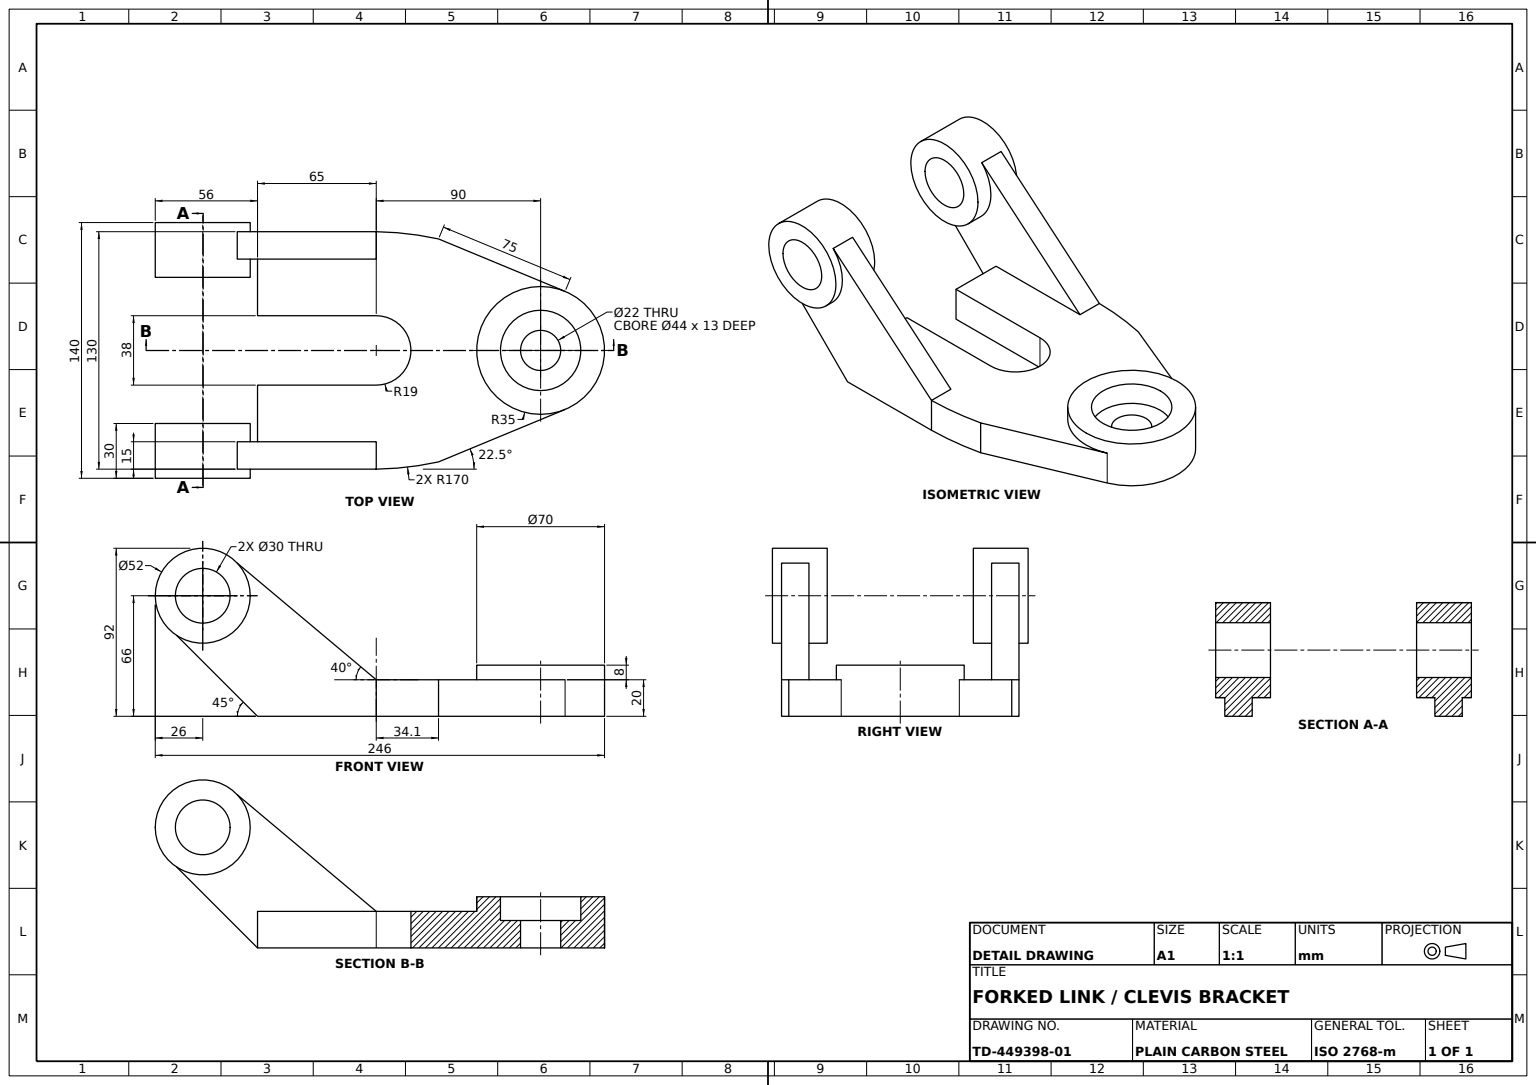
from build123d import *

# Parameters (mm, degrees)
BASE_PLATE_DEPTH           = 20
PIVOT_BOSS_SKETCH_R        = 35
PIVOT_BOSS_70_DEPTH        = 8
ARM_WEB_1_DEPTH            = 15
ARM_START                  = -15
ARM_WEB_2_DEPTH            = 15
LUG_START                  = 30
LUG_BOSS_1_SKETCH_R        = 26
LUG_BOSS_1_52_DEPTH        = 30
LUG_BOSS_2_SKETCH_R        = 26
LUG_BOSS_2_52_DEPTH        = 30
LUG_BORE_SKETCH_R          = 15
LUG_BORE_30_DEPTH          = 254.306139
PIVOT_COUNTERBORE_SKETCH_R = 22
PIVOT_COUNTERBORE_44_DEPTH = 13
PIVOT_HOLE_SKETCH_R        = 11
PIVOT_HOLE_22_DEPTH        = 224.494966


with BuildPart() as part:
    # Base Plate Sketch → Base Plate (new body)
    with BuildSketch(Plane(origin=(0, 0, 0), x_dir=(1, 0, 0), z_dir=(0, 1, 0))):
        with BuildLine():
            Line((0, 0), (0, 46))
            Line((0, 46), (65, 46))
            ThreePointArc((65, 46), (82.151777, 44.881636), (99.102955, 42.037041))
            Line((99.102955, 42.037041), (168.39392, 13.335784))
            ThreePointArc((168.39392, 13.335784), (190, -19), (168.39392, -51.335784))
            Line((168.39392, -51.335784), (99.102955, -80.037041))
            ThreePointArc((99.102955, -80.037041), (82.151777, -82.881636), (65, -84))
            Line((65, -84), (0, -84))
            Line((0, -84), (0, -38))
            Line((0, -38), (65, -38))
            ThreePointArc((65, -38), (84, -19), (65, 0))
            Line((65, 0), (0, 0))
        make_face()
    extrude(amount=BASE_PLATE_DEPTH)

    # Pivot Boss Sketch → Pivot Boss Ø70 (add)
    with BuildSketch(Plane(origin=(0, 20, 0), x_dir=(1, 0, 0), z_dir=(0, 1, 0))):
        with Locations(Location((155, -19, 0), (0, 0, 67.5))):
            Circle(PIVOT_BOSS_SKETCH_R)
    extrude(amount=PIVOT_BOSS_70_DEPTH)

    # Arm Web 1 Sketch → Arm Web 1 (add)
    with BuildSketch(Plane.XY.offset(84)):
        with BuildLine():
            Line((0, 0), (-44.258343, 44.258343))
            ThreePointArc((-44.258343, 44.258343), (-49.935425, 82.690681), (-11.103607, 83.858508))
            Line((-11.103607, 83.858508), (65, 20))
            Line((65, 20), (65, 0))
            Line((65, 0), (0, 0))
        make_face()
    extrude(amount=-ARM_WEB_1_DEPTH)

    # Arm Web 2 Sketch → Arm Web 2 (add)
    with BuildSketch(Plane(origin=(0, 0, -46), x_dir=(-1, 0, 0), z_dir=(0, 0, -1)).offset(ARM_START)):
        with BuildLine():
            Line((-65, 20), (-65, 0))
            Line((-65, 0), (0, 0))
            Line((0, 0), (44.258343, 44.258343))
            ThreePointArc((44.258343, 44.258343), (49.935425, 82.690681), (11.103607, 83.858508))
            Line((11.103607, 83.858508), (-65, 20))
        make_face()
    extrude(amount=ARM_WEB_2_DEPTH)

    # Lug Boss 1 Sketch → Lug Boss 1 Ø52 (add)
    with BuildSketch(Plane.XY.offset(-51).offset(LUG_START)):
        with Locations((-30, 66)):
            Circle(LUG_BOSS_1_SKETCH_R)
    extrude(amount=-LUG_BOSS_1_52_DEPTH)

    # Lug Boss 2 Sketch → Lug Boss 2 Ø52 (add)
    with BuildSketch(Plane.XY.offset(89)):
        with Locations((-30, 66)):
            Circle(LUG_BOSS_2_SKETCH_R)
    extrude(amount=-LUG_BOSS_2_52_DEPTH)

    # Lug Bore Sketch → Lug Bore Ø30 (cut, through all)
    with BuildSketch(Plane.XY.offset(89)):
        with Locations((-30, 66)):
            Circle(LUG_BORE_SKETCH_R)
    extrude(amount=-LUG_BORE_30_DEPTH, mode=Mode.SUBTRACT)

    # Pivot Counterbore Sketch → Pivot Counterbore Ø44 (cut)
    with BuildSketch(Plane(origin=(0, 28, 0), x_dir=(1, 0, 0), z_dir=(0, 1, 0))):
        with Locations(Location((155, -19, 0), (0, 0, 270))):
            Circle(PIVOT_COUNTERBORE_SKETCH_R)
    extrude(amount=-PIVOT_COUNTERBORE_44_DEPTH, mode=Mode.SUBTRACT)

    # Pivot Hole Sketch → Pivot Hole Ø22 (cut, through all)
    with BuildSketch(Plane(origin=(0, 15, 0), x_dir=(1, 0, 0), z_dir=(0, 1, 0))):
        with Locations(Location((155, -19, 0), (0, 0, 270))):
            Circle(PIVOT_HOLE_SKETCH_R)
    extrude(amount=-PIVOT_HOLE_22_DEPTH, mode=Mode.SUBTRACT)


solid = part.part
